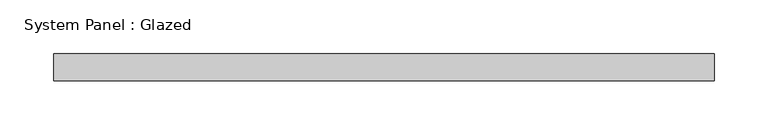
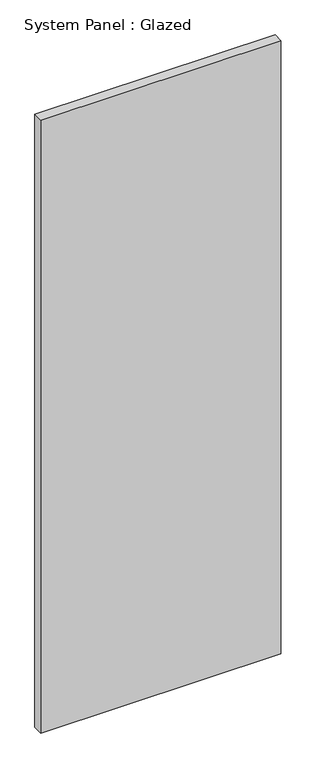
"""IFC4 building model written with IfcOpenShell, lengths in millimetres: plate geometry, System Panel : Glazed."""

from ifc_helpers import new_model, si_unit, origin, origin_with_axes, place, context, project, spatial, polyline, outline, extrude, source, transform, mapped, element, save


def system_panel_glazed_4605dce3(model_context):
    return source(origin(), model_context, "Body", "SweptSolid", [
        extrude(outline(polyline([(307.975, 19.05), (-307.975, 19.05), (-307.975, 44.45), (307.975, 44.45), (307.975, 19.05)])), origin_with_axes(), (0.0, 0.0, 1.0), 1662.0304763),
    ])


if __name__ == "__main__":
    model = new_model("IFC4")
    model_context = context("Model", 3, world=origin())
    ifc_project = project(units=[si_unit("LENGTHUNIT", "METRE", prefix="MILLI")], contexts=[model_context])
    site = spatial("IfcSite", under=ifc_project)
    building = spatial("IfcBuilding", under=site)
    placement = place(None, origin())
    system_panel_glazed_shape = system_panel_glazed_4605dce3(model_context)
    element("IfcPlate", 1, ObjectType="System Panel : Glazed", at=placement, inside=building, context=model_context, shape_type="MappedRepresentation", body=[
        mapped(system_panel_glazed_shape, transform((0.0, 0.0, 0.0), x_axis=(1.0, 0.0, 0.0), y_axis=(0.0, 1.0, 0.0), z_axis=(0.0, 0.0, 1.0))),
    ])
    save(model, "model.ifc")

# Revit data of these elements
# Type "System Panel : Glazed"
#   Construction Type Id = "GSP4R"
#   Analytic Construction = "1/8 in Pilkington single glazing"
#   Visual Light Transmittance = 0.9
#   Solar Heat Gain Coefficient = 0.86
#   Heat Transfer Coefficient (U) = 1.18115 BTU/(h·ft²·°F)
#   Define Thermal Properties by = 1
# Element 1 (IfcPlate, "System Panel : Glazed")
#   Materials on its faces: "Glass"
# Materials
#   "Glass": class "Glass", colour RGB 0 128 192, transparency 0.75, Description = "Soda Lime Glass", Cost = 0
